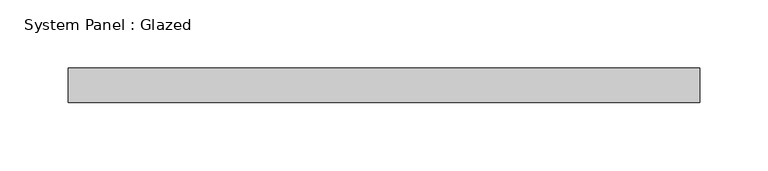
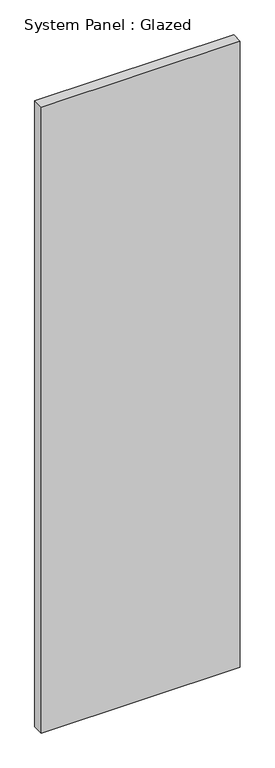
"""IFC4 building model written with IfcOpenShell, lengths in millimetres: plate geometry, System Panel : Glazed."""

from ifc_helpers import new_model, si_unit, origin, origin_with_axes, place, context, project, spatial, polyline, outline, extrude, source, transform, mapped, element, save


def system_panel_glazed_545fc278(model_context):
    return source(origin(), model_context, "Body", "SweptSolid", [
        extrude(outline(polyline([(231.775, 19.05), (-231.775, 19.05), (-231.775, 44.45), (231.775, 44.45), (231.775, 19.05)])), origin_with_axes(), (0.0, 0.0, 1.0), 1540.45282),
    ])


if __name__ == "__main__":
    model = new_model("IFC4")
    model_context = context("Model", 3, world=origin())
    ifc_project = project(units=[si_unit("LENGTHUNIT", "METRE", prefix="MILLI")], contexts=[model_context])
    site = spatial("IfcSite", under=ifc_project)
    building = spatial("IfcBuilding", under=site)
    placement = place(None, origin())
    system_panel_glazed_shape = system_panel_glazed_545fc278(model_context)
    element("IfcPlate", 1, ObjectType="System Panel : Glazed", at=placement, inside=building, context=model_context, shape_type="MappedRepresentation", body=[
        mapped(system_panel_glazed_shape, transform((0.0, 0.0, 0.0), x_axis=(1.0, 0.0, 0.0), y_axis=(0.0, 1.0, 0.0), z_axis=(0.0, 0.0, 1.0))),
    ])
    save(model, "model.ifc")

# Revit data of these elements
# Type "System Panel : Glazed"
#   Construction Type Id = "GSP4R"
#   Analytic Construction = "1/8 in Pilkington single glazing"
#   Visual Light Transmittance = 0.9
#   Solar Heat Gain Coefficient = 0.86
#   Heat Transfer Coefficient (U) = 1.18115 BTU/(h·ft²·°F)
#   Define Thermal Properties by = 1
# Element 1 (IfcPlate, "System Panel : Glazed")
#   Materials on its faces: "Glass"
# Materials
#   "Glass": class "Glass", colour RGB 0 128 192, transparency 0.75, Description = "Soda Lime Glass", Cost = 0
